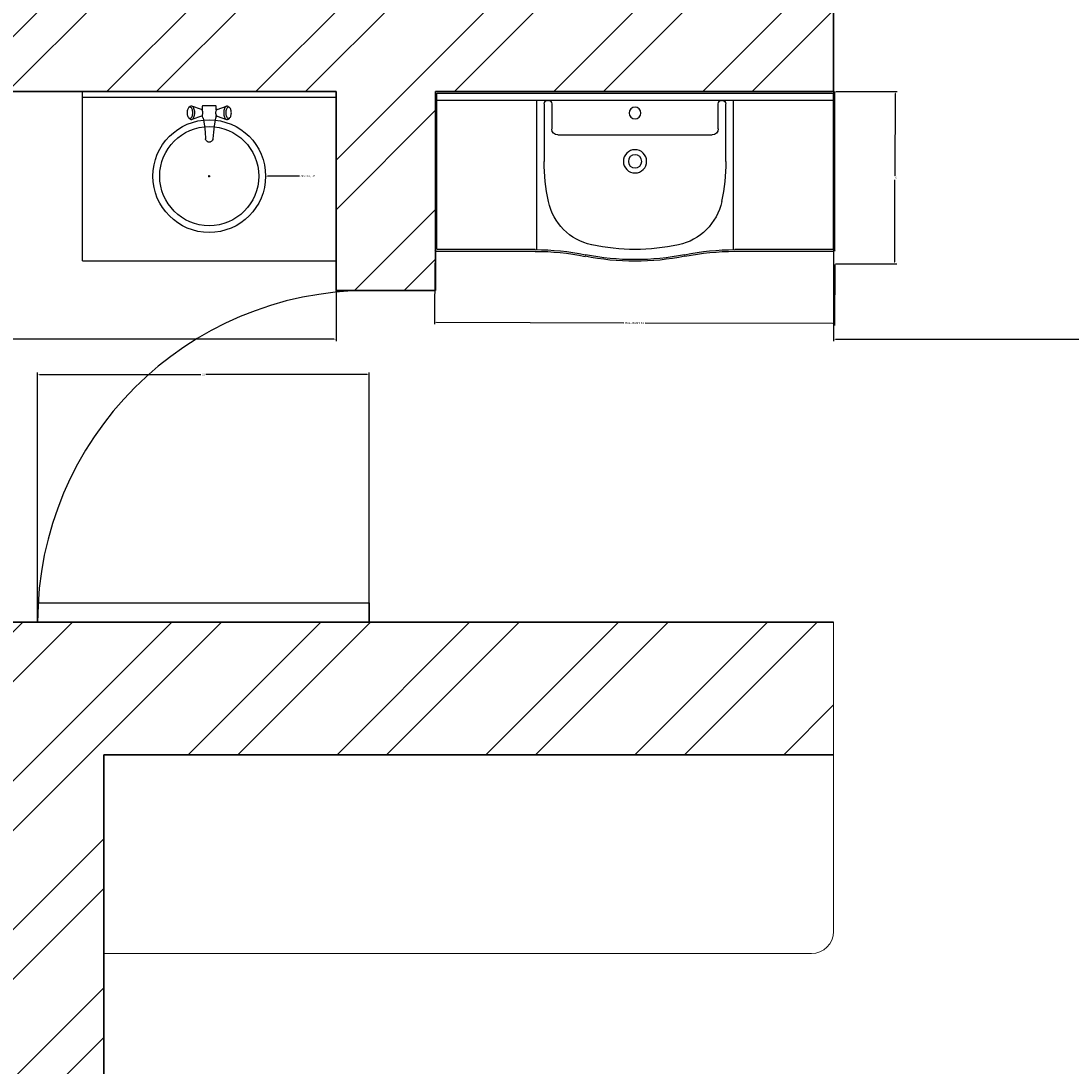
# Model space of a CAD drawing. Units: inches. Extents: x 3449 to 3843, y 1566 to 2054.
# Tile 3 of 8: x 3543 to 3638, y 1751 to 1846. Entities that reach past the tile are written whole.
import ezdxf

# ---------------------------------------------------------------- set-up
doc = ezdxf.new("R2010")
doc.units = ezdxf.units.IN
for name, color, linetype, lineweight in [('A-ANNO-DIMS', 2, 'Continuous', 18), ('A-DOOR', 4, 'Continuous', 25), ('A-FLOR-CASE', 7, 'Continuous', 20), ('A-WALL', 7, 'Continuous', 35), ('A-WALL-PATT', 251, 'Continuous', 13), ('Сантехника', 7, 'Continuous', 18)]:
    doc.layers.add(name, color=color, linetype=linetype, lineweight=lineweight)
doc.layers.add('SANTEH', color=7, linetype='Continuous')
doc.styles.get("Standard").update_dxf_attribs({"font": 'arial.ttf'})
doc.dimstyles.get("Standard").update_dxf_attribs({"dimtxt": 0.18, "dimasz": 0.18, "dimexe": 0.18, "dimexo": 0.0625, "dimgap": 0.09, "dimtad": 0, "dimtih": 1, "dimtoh": 1, "dimdec": 4, "dimzin": 0, "dimdsep": 46, "dimtxsty": 'Standard', "dimcen": 0.09, "dimadec": 0, "dimazin": 0, "dimtfac": 1, "dimtdec": 4, "dimtofl": 0, "dimtmove": 0, "dimatfit": 3, "dimfxl": 1, "dimtolj": 1, "dimtzin": 0, "dimarcsym": 0})

# ---------------------------------------------------------------- blocks, each defined once
blk = doc.blocks.new('*U6')
for p, q in [((0, 0), (0, -6)), ((30, 0), (30, -6))]:
    blk.add_line(p, q)
blk.add_lwpolyline([(0, 0), (0, 30), (1.75, 30), (1.75, 0)], close=True)
blk.add_arc((0, 0), 30, 0, 90)
blk = doc.blocks.new('Basin Built-In Circle_74')
at = {"layer": 'SANTEH'}
for p, q in [((0, 600), (900, 600)), ((0, 0), (0, 600)), ((900, 0), (900, 600)), ((0, 580), (900, 580)), ((371.7, 528.5), (371.5, 525)), ((371.7, 528.5), (371.5, 525)), ((371.5, 525), (371.7, 521.5)), ((371.5, 525), (371.7, 521.5)), ((372.1, 531.8), (371.7, 528.5)), ((372.1, 531.8), (371.7, 528.5)), ((372.8, 535), (372.1, 531.8)), ((372.8, 535), (372.1, 531.8)), ((373.8, 537.9), (372.8, 535)), ((373.8, 537.9), (372.8, 535)), ((375.1, 540.3), (373.8, 537.9)), ((375.1, 540.3), (373.8, 537.9)), ((376.5, 542.3), (375.1, 540.3)), ((376.5, 542.3), (375.1, 540.3)), ((378.1, 543.8), (376.5, 542.3)), ((378.1, 543.8), (376.5, 542.3)), ((382.6, 547.6), (378.1, 543.8)), ((382.6, 547.6), (378.1, 543.8)), ((379.8, 544.7), (378.1, 543.8)), ((379.8, 544.7), (378.1, 543.8)), ((381.5, 545), (379.8, 544.7)), ((381.5, 545), (379.8, 544.7)), ((383.2, 544.7), (381.5, 545)), ((383.2, 544.7), (381.5, 545)), ((384.6, 548.6), (382.6, 547.6)), ((384.6, 548.6), (382.6, 547.6)), ((384.9, 543.8), (383.2, 544.7)), ((384.9, 543.8), (383.2, 544.7)), ((386.7, 549), (384.6, 548.6)), ((386.7, 549), (384.6, 548.6)), ((386.5, 542.3), (384.9, 543.8)), ((386.5, 542.3), (384.9, 543.8)), ((387.9, 540.3), (386.5, 542.3)), ((387.9, 540.3), (386.5, 542.3)), ((388.8, 548.6), (386.7, 549)), ((388.8, 548.6), (386.7, 549)), ((389.2, 537.9), (387.9, 540.3)), ((389.2, 537.9), (387.9, 540.3)), ((390.8, 547.6), (388.8, 548.6)), ((422.4, 536.8), (388.8, 548.6)), ((390.8, 547.6), (388.8, 548.6)), ((422.4, 536.8), (388.8, 548.6)), ((390.2, 535), (389.2, 537.9)), ((390.2, 535), (389.2, 537.9)), ((390.9, 531.8), (390.2, 535)), ((390.9, 531.8), (390.2, 535)), ((392.7, 545.8), (390.8, 547.6)), ((392.7, 545.8), (390.8, 547.6)), ((391.4, 528.5), (390.9, 531.8)), ((391.4, 528.5), (390.9, 531.8)), ((391.5, 525), (391.4, 528.5)), ((391.5, 525), (391.4, 528.5)), ((391.4, 521.5), (391.5, 525)), ((391.4, 521.5), (391.5, 525)), ((394.4, 543.4), (392.7, 545.8)), ((394.4, 543.4), (392.7, 545.8)), ((395.9, 540.4), (394.4, 543.4)), ((395.9, 540.4), (394.4, 543.4)), ((397.1, 537), (395.9, 540.4)), ((397.1, 537), (395.9, 540.4)), ((398, 533.2), (397.1, 537)), ((398, 533.2), (397.1, 537)), ((398.5, 529.2), (398, 533.2)), ((398.5, 529.2), (398, 533.2)), ((398.7, 525), (398.5, 529.2)), ((398.7, 525), (398.5, 529.2)), ((398.5, 520.8), (398.7, 525)), ((398.5, 520.8), (398.7, 525)), ((423.4, 536.3), (422.4, 536.8)), ((423.4, 536.3), (422.4, 536.8)), ((424.3, 535.4), (423.4, 536.3)), ((424.3, 535.4), (423.4, 536.3)), ((425.2, 534.2), (424.3, 535.4)), ((425.2, 534.2), (424.3, 535.4)), ((426.7, 535), (424.6, 535)), ((426.7, 535), (424.6, 535)), ((425.2, 548), (425, 547.5)), ((425.2, 548), (425, 547.5)), ((425, 547.5), (425, 547)), ((425, 547.5), (425, 547)), ((425, 547), (425, 535)), ((425, 547), (425, 535)), ((425.4, 548.5), (425.2, 548)), ((425.4, 548.5), (425.2, 548)), ((425.9, 532.7), (425.2, 534.2)), ((425.9, 532.7), (425.2, 534.2)), ((425.7, 548.9), (425.4, 548.5)), ((425.7, 548.9), (425.4, 548.5)), ((426.1, 549.3), (425.7, 548.9)), ((426.1, 549.3), (425.7, 548.9)), ((426.5, 531), (425.9, 532.7)), ((426.5, 531), (425.9, 532.7)), ((426.5, 549.6), (426.1, 549.3)), ((426.5, 549.6), (426.1, 549.3)), ((427, 549.8), (426.5, 549.6)), ((427, 549.8), (426.5, 549.6)), ((427, 529.1), (426.5, 531)), ((427, 529.1), (426.5, 531)), ((427.5, 550), (427, 549.8)), ((427.5, 550), (427, 549.8)), ((427.2, 527.1), (427, 529.1)), ((427.2, 527.1), (427, 529.1)), ((427, 520.9), (427.2, 522.9)), ((427, 520.9), (427.2, 522.9)), ((427.3, 525), (427.2, 527.1)), ((427.3, 525), (427.2, 527.1)), ((427.2, 522.9), (427.3, 525)), ((427.2, 522.9), (427.3, 525)), ((428, 550), (427.5, 550)), ((428, 550), (427.5, 550)), ((472, 550), (428, 550)), ((472, 550), (428, 550)), ((472.5, 550), (472, 550)), ((472.5, 550), (472, 550)), ((473, 549.8), (472.5, 550)), ((473, 549.8), (472.5, 550)), ((472.8, 527.1), (472.7, 525)), ((472.8, 527.1), (472.7, 525)), ((472.7, 525), (472.8, 522.9)), ((472.7, 525), (472.8, 522.9)), ((473, 529.1), (472.8, 527.1)), ((473, 529.1), (472.8, 527.1)), ((472.8, 522.9), (473, 520.9)), ((472.8, 522.9), (473, 520.9)), ((473.5, 549.6), (473, 549.8)), ((473.5, 549.6), (473, 549.8)), ((473.5, 531), (473, 529.1)), ((473.5, 531), (473, 529.1)), ((473.9, 549.3), (473.5, 549.6)), ((473.9, 549.3), (473.5, 549.6)), ((475.4, 535), (473.5, 535)), ((475.4, 535), (473.5, 535)), ((474.1, 532.7), (473.5, 531)), ((474.1, 532.7), (473.5, 531)), ((474.3, 548.9), (473.9, 549.3)), ((474.3, 548.9), (473.9, 549.3)), ((474.8, 534.2), (474.1, 532.7)), ((474.8, 534.2), (474.1, 532.7)), ((474.6, 548.5), (474.3, 548.9)), ((474.6, 548.5), (474.3, 548.9)), ((474.8, 548), (474.6, 548.5)), ((474.8, 548), (474.6, 548.5)), ((475, 547.5), (474.8, 548)), ((475, 547.5), (474.8, 548)), ((475.7, 535.4), (474.8, 534.2)), ((475.7, 535.4), (474.8, 534.2)), ((475, 547), (475, 547.5)), ((475, 547), (475, 547.5)), ((475, 535), (475, 547)), ((475, 535), (475, 547)), ((476.6, 536.3), (475.7, 535.4)), ((476.6, 536.3), (475.7, 535.4)), ((477.6, 536.8), (476.6, 536.3)), ((477.6, 536.8), (476.6, 536.3)), ((477.6, 536.8), (511.2, 548.6)), ((477.6, 536.8), (511.2, 548.6)), ((501.5, 529.2), (501.3, 525)), ((501.5, 529.2), (501.3, 525)), ((501.3, 525), (501.5, 520.8)), ((501.3, 525), (501.5, 520.8)), ((502, 533.2), (501.5, 529.2)), ((502, 533.2), (501.5, 529.2)), ((502.9, 537), (502, 533.2)), ((502.9, 537), (502, 533.2)), ((504.1, 540.4), (502.9, 537)), ((504.1, 540.4), (502.9, 537)), ((505.6, 543.4), (504.1, 540.4)), ((505.6, 543.4), (504.1, 540.4)), ((507.3, 545.8), (505.6, 543.4)), ((507.3, 545.8), (505.6, 543.4)), ((509.2, 547.6), (507.3, 545.8)), ((509.2, 547.6), (507.3, 545.8)), ((508.6, 528.5), (508.5, 525)), ((508.6, 528.5), (508.5, 525)), ((508.5, 525), (508.6, 521.5)), ((508.5, 525), (508.6, 521.5)), ((509.1, 531.8), (508.6, 528.5)), ((509.1, 531.8), (508.6, 528.5)), ((509.8, 535), (509.1, 531.8)), ((509.8, 535), (509.1, 531.8)), ((511.2, 548.6), (509.2, 547.6)), ((511.2, 548.6), (509.2, 547.6)), ((510.8, 537.9), (509.8, 535)), ((510.8, 537.9), (509.8, 535)), ((512.1, 540.3), (510.8, 537.9)), ((512.1, 540.3), (510.8, 537.9)), ((513.3, 549), (511.2, 548.6)), ((513.3, 549), (511.2, 548.6)), ((513.5, 542.3), (512.1, 540.3)), ((513.5, 542.3), (512.1, 540.3)), ((515.4, 548.6), (513.3, 549)), ((515.4, 548.6), (513.3, 549)), ((515.1, 543.8), (513.5, 542.3)), ((515.1, 543.8), (513.5, 542.3)), ((516.8, 544.7), (515.1, 543.8)), ((516.8, 544.7), (515.1, 543.8)), ((517.4, 547.6), (515.4, 548.6)), ((517.4, 547.6), (515.4, 548.6)), ((518.5, 545), (516.8, 544.7)), ((518.5, 545), (516.8, 544.7)), ((517.4, 547.6), (521.9, 543.8)), ((517.4, 547.6), (521.9, 543.8)), ((520.2, 544.7), (518.5, 545)), ((520.2, 544.7), (518.5, 545)), ((521.9, 543.8), (520.2, 544.7)), ((521.9, 543.8), (520.2, 544.7)), ((523.5, 542.3), (521.9, 543.8)), ((523.5, 542.3), (521.9, 543.8)), ((524.9, 540.3), (523.5, 542.3)), ((524.9, 540.3), (523.5, 542.3)), ((526.2, 537.9), (524.9, 540.3)), ((526.2, 537.9), (524.9, 540.3)), ((527.2, 535), (526.2, 537.9)), ((527.2, 535), (526.2, 537.9)), ((527.9, 531.8), (527.2, 535)), ((527.9, 531.8), (527.2, 535)), ((528.3, 528.5), (527.9, 531.8)), ((528.3, 528.5), (527.9, 531.8)), ((528.5, 525), (528.3, 528.5)), ((528.5, 525), (528.3, 528.5)), ((528.3, 521.5), (528.5, 525)), ((528.3, 521.5), (528.5, 525)), ((371.7, 521.5), (372.1, 518.2)), ((371.7, 521.5), (372.1, 518.2)), ((372.1, 518.2), (372.8, 515)), ((372.1, 518.2), (372.8, 515)), ((372.8, 515), (373.8, 512.1)), ((372.8, 515), (373.8, 512.1)), ((373.8, 512.1), (375.1, 509.7)), ((373.8, 512.1), (375.1, 509.7)), ((375.1, 509.7), (376.5, 507.7)), ((375.1, 509.7), (376.5, 507.7)), ((376.5, 507.7), (378.1, 506.2)), ((376.5, 507.7), (378.1, 506.2)), ((378.1, 506.2), (379.8, 505.3)), ((382.6, 502.4), (378.1, 506.2)), ((378.1, 506.2), (379.8, 505.3)), ((382.6, 502.4), (378.1, 506.2)), ((379.8, 505.3), (381.5, 505)), ((379.8, 505.3), (381.5, 505)), ((381.5, 505), (383.2, 505.3)), ((381.5, 505), (383.2, 505.3)), ((382.6, 502.4), (384.6, 501.4)), ((382.6, 502.4), (384.6, 501.4)), ((383.2, 505.3), (384.9, 506.2)), ((383.2, 505.3), (384.9, 506.2)), ((384.6, 501.4), (386.7, 501)), ((384.6, 501.4), (386.7, 501)), ((384.9, 506.2), (386.5, 507.7)), ((384.9, 506.2), (386.5, 507.7)), ((386.5, 507.7), (387.9, 509.7)), ((386.5, 507.7), (387.9, 509.7)), ((386.7, 501), (388.8, 501.4)), ((386.7, 501), (388.8, 501.4)), ((387.9, 509.7), (389.2, 512.1)), ((387.9, 509.7), (389.2, 512.1)), ((422.4, 513.2), (388.8, 501.4)), ((422.4, 513.2), (388.8, 501.4)), ((388.8, 501.4), (390.8, 502.4)), ((388.8, 501.4), (390.8, 502.4)), ((389.2, 512.1), (390.2, 515)), ((389.2, 512.1), (390.2, 515)), ((390.2, 515), (390.9, 518.2)), ((390.2, 515), (390.9, 518.2)), ((390.8, 502.4), (392.7, 504.2)), ((390.8, 502.4), (392.7, 504.2)), ((390.9, 518.2), (391.4, 521.5)), ((390.9, 518.2), (391.4, 521.5)), ((392.7, 504.2), (394.4, 506.6)), ((392.7, 504.2), (394.4, 506.6)), ((394.4, 506.6), (395.9, 509.6)), ((394.4, 506.6), (395.9, 509.6)), ((395.9, 509.6), (397.1, 513)), ((395.9, 509.6), (397.1, 513)), ((397.1, 513), (398, 516.8)), ((397.1, 513), (398, 516.8)), ((398, 516.8), (398.5, 520.8)), ((398, 516.8), (398.5, 520.8)), ((422.4, 513.2), (423.4, 513.7)), ((422.4, 513.2), (423.4, 513.7)), ((423.4, 513.7), (424.3, 514.6)), ((423.4, 513.7), (424.3, 514.6)), ((424.3, 514.6), (425.2, 515.8)), ((424.3, 514.6), (425.2, 515.8)), ((427.1, 515), (424.6, 515)), ((427.1, 515), (424.6, 515)), ((425, 515), (425, 513)), ((425, 515), (425, 513)), ((425, 513), (425, 512.5)), ((425, 513), (425, 512.5)), ((425, 512.5), (425.2, 512)), ((425, 512.5), (425.2, 512)), ((425.2, 515.8), (425.9, 517.3)), ((425.2, 515.8), (425.9, 517.3)), ((425.2, 512), (428.1, 505.1)), ((425.2, 512), (428.1, 505.1)), ((425.9, 517.3), (426.5, 519)), ((425.9, 517.3), (426.5, 519)), ((426.5, 519), (427, 520.9)), ((426.5, 519), (427, 520.9)), ((428, 505.4), (430.7, 493.4)), ((428, 505.4), (430.7, 493.4)), ((430.7, 493.4), (433, 477.1)), ((430.7, 493.4), (433, 477.1)), ((469.3, 493.4), (467, 477.1)), ((469.3, 493.4), (467, 477.1)), ((472, 505.4), (469.3, 493.4)), ((472, 505.4), (469.3, 493.4)), ((474.8, 512), (471.9, 505.1)), ((474.8, 512), (471.9, 505.1)), ((473, 520.9), (473.5, 519)), ((473, 520.9), (473.5, 519)), ((475.4, 515), (473.2, 515)), ((475.4, 515), (473.2, 515)), ((473.5, 519), (474.1, 517.3)), ((473.5, 519), (474.1, 517.3)), ((474.1, 517.3), (474.8, 515.8)), ((474.1, 517.3), (474.8, 515.8)), ((474.8, 515.8), (475.7, 514.6)), ((474.8, 515.8), (475.7, 514.6)), ((474.8, 512), (475, 512.5)), ((474.8, 512), (475, 512.5)), ((475, 513), (475, 515)), ((475, 513), (475, 515)), ((475, 512.5), (475, 513)), ((475, 512.5), (475, 513)), ((475.7, 514.6), (476.6, 513.7)), ((475.7, 514.6), (476.6, 513.7)), ((476.6, 513.7), (477.6, 513.2)), ((476.6, 513.7), (477.6, 513.2)), ((477.6, 513.2), (511.2, 501.4)), ((477.6, 513.2), (511.2, 501.4)), ((501.5, 520.8), (502, 516.8)), ((501.5, 520.8), (502, 516.8)), ((502, 516.8), (502.9, 513)), ((502, 516.8), (502.9, 513)), ((502.9, 513), (504.1, 509.6)), ((502.9, 513), (504.1, 509.6)), ((504.1, 509.6), (505.6, 506.6)), ((504.1, 509.6), (505.6, 506.6)), ((505.6, 506.6), (507.3, 504.2)), ((505.6, 506.6), (507.3, 504.2)), ((507.3, 504.2), (509.2, 502.4)), ((507.3, 504.2), (509.2, 502.4)), ((508.6, 521.5), (509.1, 518.2)), ((508.6, 521.5), (509.1, 518.2)), ((509.1, 518.2), (509.8, 515)), ((509.1, 518.2), (509.8, 515)), ((509.2, 502.4), (511.2, 501.4)), ((509.2, 502.4), (511.2, 501.4)), ((509.8, 515), (510.8, 512.1)), ((509.8, 515), (510.8, 512.1)), ((510.8, 512.1), (512.1, 509.7)), ((510.8, 512.1), (512.1, 509.7)), ((511.2, 501.4), (513.3, 501)), ((511.2, 501.4), (513.3, 501)), ((512.1, 509.7), (513.5, 507.7)), ((512.1, 509.7), (513.5, 507.7)), ((513.3, 501), (515.4, 501.4)), ((513.3, 501), (515.4, 501.4)), ((513.5, 507.7), (515.1, 506.2)), ((513.5, 507.7), (515.1, 506.2)), ((515.1, 506.2), (516.8, 505.3)), ((515.1, 506.2), (516.8, 505.3)), ((515.4, 501.4), (517.4, 502.4)), ((515.4, 501.4), (517.4, 502.4)), ((516.8, 505.3), (518.5, 505)), ((516.8, 505.3), (518.5, 505)), ((517.4, 502.4), (521.9, 506.2)), ((517.4, 502.4), (521.9, 506.2)), ((518.5, 505), (520.2, 505.3)), ((518.5, 505), (520.2, 505.3)), ((520.2, 505.3), (521.9, 506.2)), ((520.2, 505.3), (521.9, 506.2)), ((521.9, 506.2), (523.5, 507.7)), ((521.9, 506.2), (523.5, 507.7)), ((523.5, 507.7), (524.9, 509.7)), ((523.5, 507.7), (524.9, 509.7)), ((524.9, 509.7), (526.2, 512.1)), ((524.9, 509.7), (526.2, 512.1)), ((526.2, 512.1), (527.2, 515)), ((526.2, 512.1), (527.2, 515)), ((527.2, 515), (527.9, 518.2)), ((527.2, 515), (527.9, 518.2)), ((527.9, 518.2), (528.3, 521.5)), ((527.9, 518.2), (528.3, 521.5)), ((433, 477.2), (435, 456.1)), ((433, 477.2), (435, 456.1)), ((435, 456.1), (436.8, 432.9)), ((435, 456.1), (436.8, 432.9)), ((465, 456.1), (463.2, 432.9)), ((465, 456.1), (463.2, 432.9)), ((467, 477.2), (465, 456.1)), ((467, 477.2), (465, 456.1)), ((437, 430.8), (436.8, 432.9)), ((437, 430.8), (436.8, 432.9)), ((437, 430.7), (437, 430.8)), ((437, 430.7), (437, 430.8)), ((437.6, 428.7), (437, 430.7)), ((437.6, 428.7), (437, 430.7)), ((438.6, 426.9), (437.6, 428.7)), ((438.6, 426.9), (437.6, 428.7)), ((440, 425.1), (438.6, 426.9)), ((440, 425.1), (438.6, 426.9)), ((441.6, 423.7), (440, 425.1)), ((441.6, 423.7), (440, 425.1)), ((443.5, 422.5), (441.6, 423.7)), ((443.5, 422.5), (441.6, 423.7)), ((445.6, 421.7), (443.5, 422.5)), ((445.6, 421.7), (443.5, 422.5)), ((445, 421.7), (443.9, 422.4)), ((446.6, 421), (445, 421.7)), ((447.7, 421.2), (445.6, 421.7)), ((447.7, 421.2), (445.6, 421.7)), ((448.3, 420.6), (446.6, 421)), ((450, 421), (447.7, 421.2)), ((450, 421), (447.7, 421.2)), ((450, 420.5), (448.3, 420.6)), ((452.3, 421.2), (450, 421)), ((452.3, 421.2), (450, 421)), ((451.7, 420.6), (450, 420.5)), ((453.4, 421), (451.7, 420.6)), ((454.4, 421.7), (452.3, 421.2)), ((454.4, 421.7), (452.3, 421.2)), ((455, 421.7), (453.4, 421)), ((456.5, 422.5), (454.4, 421.7)), ((456.5, 422.5), (454.4, 421.7)), ((456.1, 422.4), (455, 421.7)), ((458.4, 423.7), (456.5, 422.5)), ((458.4, 423.7), (456.5, 422.5)), ((460, 425.1), (458.4, 423.7)), ((460, 425.1), (458.4, 423.7)), ((461.4, 426.9), (460, 425.1)), ((461.4, 426.9), (460, 425.1)), ((462.4, 428.7), (461.4, 426.9)), ((462.4, 428.7), (461.4, 426.9)), ((463, 430.7), (462.4, 428.7)), ((463, 430.7), (462.4, 428.7)), ((463.2, 432.9), (463, 430.8)), ((463.2, 432.9), (463, 430.8)), ((463, 430.7), (463, 430.8)), ((463, 430.7), (463, 430.8)), ((0, 0), (900, 0))]:
    blk.add_line(p, q, dxfattribs=at)
for radius in [200, 175.8]:
    blk.add_circle((450, 300), radius, dxfattribs=at)
blk = doc.blocks.new('s_02')
at = {"layer": 'SANTEH'}
for p, q in [((0, 0), (-519.4, -1.7)), ((0, 0), (-519.4, -1.7)), ((-520.5, -2.8), (-519.8, -209.5)), ((-520.5, -2.8), (-519.8, -209.5)), ((-517.6, -207.3), (-518.3, -5)), ((-1, -11.7), (-518.3, -13.5)), ((-517.2, -3.9), (-2.2, -2.2)), ((-387.2, -207.9), (-387.9, -13)), ((-131.4, -12.2), (-130.8, -207.1)), ((-1.1, -3.3), (-0.4, -205.6)), ((1.8, -207.7), (1.1, -1.1)), ((1.8, -207.7), (1.1, -1.1)), ((-378.3, -17.4), (-378.1, -92.6)), ((-368.3, -17.3), (-368.2, -50.3)), ((-150.9, -49.6), (-151, -16.6)), ((-140.7, -91.8), (-141, -16.6)), ((-360.4, -58.1), (-158.7, -57.4)), ((-518.7, -210.5), (-389.4, -210.1)), ((-518.7, -210.5), (-389.4, -210.1)), ((-389.4, -207.9), (-516.6, -208.4)), ((-1.5, -206.6), (-128.6, -207.1)), ((-128.6, -209.2), (0.7, -208.8)), ((-128.6, -209.2), (0.7, -208.8))]:
    blk.add_line(p, q, dxfattribs=at)
at = {"layer": 'SANTEH', "extrusion": (0, 0, -1)}
for centre, major_axis, ratio, start_param, end_param in [((0, -1.1), (-0.38, 1.02), 0.991976, 0.357514, 1.923061), ((0, -1.1), (-0.38, 1.02), 0.991976, 0.357514, 1.923061), ((-519.4, -2.8), (0, -1.09), 0.99914, 1.570796, 3.141593), ((-519.4, -2.8), (0, -1.09), 0.99914, 1.570796, 3.141593), ((-517.2, -5), (0, -1.09), 0.99914, 1.570796, 3.141593), ((-374, -17.3), (0.01, -4.35), 0.99914, 1.570796, 3.141593), ((-372.7, -17.3), (0.01, -4.35), 0.99914, 3.141593, 4.712389), ((-146.6, -16.6), (0.01, -4.35), 0.99914, 1.570796, 3.141593), ((-145.3, -16.6), (0.01, -4.35), 0.99914, 3.141593, 4.712389), ((-2.2, -3.3), (0, -1.09), 0.99914, 3.141593, 4.712389), ((-259.6, -29.1), (0.03, -7.61), 0.99914, 1.570796326742688, 7.853981633922275), ((-360.4, -50.3), (0.03, -7.83), 0.99914, 0, 1.570796), ((-158.7, -49.6), (0.03, -7.83), 0.99914, -1.570796, 0), ((-259.4, -92.2), (0.1, -15.2), 0.99914, 1.570796326791235, 7.853981633970821), ((-128, -91.8), (0.8, -250.2), 0.99914, 1.359365, 1.570796), ((-259.4, -92.2), (0.03, -8.7), 0.99914, 1.570796326873691, 7.853981634053277), ((-390.8, -92.7), (0.8, -250.2), 0.99914, -1.570796, -1.359365), ((-300.4, -129.4), (0.2, -73.7), 0.99914, 0.211723, 1.359365), ((-218.1, -129.1), (0.2, -73.7), 0.99914, -1.359365, -0.211723), ((-259.9, 62.3), (0.9, -269.6), 0.99914, -0.211723, 0.211723), ((-1.5, -205.6), (0, -1.09), 0.99914, 4.712389, 6.283185), ((-518.7, -209.5), (0, -1.09), 0.99914, 0, 1.570796), ((-518.7, -209.5), (0, -1.09), 0.99914, 0, 1.570796), ((-516.6, -207.3), (0, -1.09), 0.99914, 0, 1.570796), ((-388.3, -539.7), (1.1, -331.7), 0.99914, 3.141593, 3.34093), ((-388.3, -539.7), (1.1, -329.5), 0.99914, 3.141593, 3.34093), ((-388.3, -539.7), (1.1, -329.5), 0.99914, 3.141593, 3.34093), ((-260.1, 106.8), (1.1, -329.5), 0.99914, -0.199337, 0.199337), ((-260.1, 106.8), (1.1, -329.5), 0.99914, -0.199337, 0.199337), ((-260.1, 106.8), (1.1, -327.4), 0.99914, -0.199337, 0.199337), ((-127.5, -538.8), (1.1, -331.7), 0.99914, 2.942255, 3.141593), ((-127.5, -538.8), (1.1, -329.5), 0.99914, 2.942255, 3.141593), ((-127.5, -538.8), (1.1, -329.5), 0.99914, 2.942255, 3.141593), ((0.7, -207.7), (0, -1.09), 0.99914, 4.712389, 6.283185), ((0.7, -207.7), (0, -1.09), 0.99914, 4.712389, 6.283185)]:
    blk.add_ellipse(centre, major_axis=major_axis, ratio=ratio, start_param=start_param, end_param=end_param, dxfattribs=at)
blk = doc.blocks.new('*D64')
at = {"layer": 'A-ANNO-DIMS', "color": 0, "lineweight": -2, "transparency": 16777216}
for p, q in [((3580.014, 1824.107), (3579.996, 1818.561)), ((3616.2, 1823.986), (3616.181, 1818.441)), ((3580.176, 1818.741), (3597.113, 1818.684)), ((3616.002, 1818.621), (3599.065, 1818.678))]:
    blk.add_line(p, q, dxfattribs=at)
at = {"layer": 'A-ANNO-DIMS', "color": 0, "transparency": 16777216}
for points in [[(3580.177, 1818.771), (3580.176, 1818.711), (3579.996, 1818.741)], [(3616.002, 1818.651), (3616.002, 1818.591), (3616.182, 1818.621)]]:
    blk.add_solid(points, dxfattribs=at)
at = {"layer": 'Defpoints', "color": 0, "transparency": 16777216}
for p in [(3580.015, 1824.169), (3616.2, 1824.048), (3616.182, 1818.621)]:
    blk.add_point(p, dxfattribs=at)
at = {"layer": 'A-ANNO-DIMS', "color": 0, "transparency": 16777216, "insert": (3598.089, 1818.681), "char_height": 0.18, "attachment_point": 5}
blk.add_mtext('\\A1;HALL BASIN 36', dxfattribs=at)
blk = doc.blocks.new('*D65')
at = {"layer": 'A-ANNO-DIMS', "color": 0, "lineweight": -2, "transparency": 16777216}
for p, q in [((3616.314, 1839.636), (3621.86, 1839.617)), ((3621.679, 1839.438), (3621.654, 1832.006)), ((3621.628, 1824.21), (3621.653, 1831.642)), ((3616.262, 1824.048), (3621.808, 1824.03))]:
    blk.add_line(p, q, dxfattribs=at)
at = {"layer": 'A-ANNO-DIMS', "color": 0, "transparency": 16777216}
for points in [[(3621.649, 1839.438), (3621.709, 1839.438), (3621.68, 1839.618)], [(3621.598, 1824.21), (3621.658, 1824.21), (3621.628, 1824.03)]]:
    blk.add_solid(points, dxfattribs=at)
at = {"layer": 'Defpoints', "color": 0, "transparency": 16777216}
for p in [(3616.252, 1839.636), (3621.68, 1839.618), (3616.2, 1824.048)]:
    blk.add_point(p, dxfattribs=at)
at = {"layer": 'A-ANNO-DIMS', "color": 0, "transparency": 16777216, "insert": (3621.654, 1831.824), "char_height": 0.18, "attachment_point": 5}
blk.add_mtext('\\A1;16', dxfattribs=at)
blk = doc.blocks.new('*D89')
at = {"layer": 'A-ANNO-DIMS', "color": 0, "lineweight": -2, "transparency": 16777216}
for p, q in [((3481.088, 1839.552), (3481.088, 1817.034)), ((3571.088, 1839.552), (3571.088, 1817.034)), ((3481.268, 1817.214), (3525.869, 1817.214)), ((3570.908, 1817.214), (3526.307, 1817.214))]:
    blk.add_line(p, q, dxfattribs=at)
at = {"layer": 'A-ANNO-DIMS', "color": 0, "transparency": 16777216}
for points in [[(3481.268, 1817.244), (3481.268, 1817.184), (3481.088, 1817.214)], [(3570.908, 1817.244), (3570.908, 1817.184), (3571.088, 1817.214)]]:
    blk.add_solid(points, dxfattribs=at)
at = {"layer": 'Defpoints', "color": 0, "transparency": 16777216}
for p in [(3481.088, 1839.614), (3571.088, 1839.614), (3481.088, 1817.214)]:
    blk.add_point(p, dxfattribs=at)
at = {"layer": 'A-ANNO-DIMS', "color": 0, "transparency": 16777216, "insert": (3526.088, 1817.214), "char_height": 0.18, "attachment_point": 5}
blk.add_mtext('\\A1;90', dxfattribs=at)
blk = doc.blocks.new('*D94')
at = {"layer": 'A-ANNO-DIMS', "color": 0, "lineweight": -2, "transparency": 16777216}
for p, q in [((3616.088, 1839.552), (3616.088, 1817.034)), ((3664.088, 1839.552), (3664.088, 1817.034)), ((3616.268, 1817.214), (3639.865, 1817.214)), ((3663.908, 1817.214), (3640.311, 1817.214))]:
    blk.add_line(p, q, dxfattribs=at)
at = {"layer": 'A-ANNO-DIMS', "color": 0, "transparency": 16777216}
for points in [[(3616.268, 1817.244), (3616.268, 1817.184), (3616.088, 1817.214)], [(3663.908, 1817.244), (3663.908, 1817.184), (3664.088, 1817.214)]]:
    blk.add_solid(points, dxfattribs=at)
at = {"layer": 'Defpoints', "color": 0, "transparency": 16777216}
for p in [(3616.088, 1839.614), (3664.088, 1839.614), (3616.088, 1817.214)]:
    blk.add_point(p, dxfattribs=at)
at = {"layer": 'A-ANNO-DIMS', "color": 0, "transparency": 16777216, "insert": (3640.088, 1817.214), "char_height": 0.18, "attachment_point": 5}
blk.add_mtext('\\A1;48', dxfattribs=at)
blk = doc.blocks.new('*D111')
at = {"layer": 'A-ANNO-DIMS', "color": 0, "lineweight": -2, "transparency": 16777216}
for p, q in [((3544.088, 1791.677), (3544.088, 1814.194)), ((3544.268, 1814.014), (3558.869, 1814.014)), ((3573.908, 1814.014), (3559.307, 1814.014)), ((3574.088, 1791.677), (3574.088, 1814.194))]:
    blk.add_line(p, q, dxfattribs=at)
at = {"layer": 'A-ANNO-DIMS', "color": 0, "transparency": 16777216}
for points in [[(3544.268, 1814.044), (3544.268, 1813.984), (3544.088, 1814.014)], [(3573.908, 1814.044), (3573.908, 1813.984), (3574.088, 1814.014)]]:
    blk.add_solid(points, dxfattribs=at)
at = {"layer": 'Defpoints', "color": 0, "transparency": 16777216}
for p in [(3574.088, 1814.014), (3544.088, 1791.614), (3574.088, 1791.614)]:
    blk.add_point(p, dxfattribs=at)
at = {"layer": 'A-ANNO-DIMS', "color": 0, "transparency": 16777216, "insert": (3559.088, 1814.014), "char_height": 0.18, "attachment_point": 5}
blk.add_mtext('\\A1;30', dxfattribs=at)
blk = doc.blocks.new('*D127')
at = {"layer": 'A-ANNO-DIMS', "color": 0, "lineweight": -2, "transparency": 16777216}
for p, q in [((3559.527, 1831.967), (3559.707, 1831.967)), ((3559.617, 1831.877), (3559.617, 1832.057)), ((3567.774, 1831.967), (3564.895, 1831.967))]:
    blk.add_line(p, q, dxfattribs=at)
at = {"layer": 'A-ANNO-DIMS', "color": 0, "transparency": 16777216}
blk.add_solid([(3564.895, 1831.997), (3564.895, 1831.937), (3564.715, 1831.967)], dxfattribs=at)
at = {"layer": 'Defpoints', "color": 0, "transparency": 16777216}
for p in [(3554.518, 1831.967), (3564.715, 1831.967)]:
    blk.add_point(p, dxfattribs=at)
at = {"layer": 'A-ANNO-DIMS', "color": 0, "transparency": 16777216, "insert": (3568.526, 1831.967), "char_height": 0.18, "attachment_point": 5}
blk.add_mtext('\\A1;2X ∅10.197', dxfattribs=at)

msp = doc.modelspace()

# ---------------------------------------------------------------- hatches: boundary and pattern name
at = {"layer": 'A-WALL-PATT'}
h = msp.add_hatch(dxfattribs=at)
h.set_pattern_fill('ANSI32', color=256)
edge = h.paths.add_edge_path()
edge.add_line((3481.088, 2022.6144), (3508.088, 2022.6144))
edge.add_line((3508.088, 2022.6144), (3508.088, 2031.6144))
edge.add_line((3508.088, 2031.6144), (3472.088, 2031.6144))
edge.add_line((3472.088, 2031.6144), (3472.088, 1779.6144))
edge.add_line((3472.088, 1779.6144), (3481.088, 1779.6144))
edge.add_line((3481.088, 1779.6144), (3481.088, 1839.6144))
edge.add_line((3481.088, 1839.6144), (3571.088, 1839.6144))
edge.add_line((3571.088, 1839.6144), (3571.088, 1824.3194))
edge.add_line((3571.088, 1824.3194), (3571.088, 1821.6144))
edge.add_line((3571.088, 1821.6144), (3580.088, 1821.6144))
edge.add_line((3580.088, 1821.6144), (3580.088, 1825.1908))
edge.add_ellipse((3580.1411, 1825.2442), major_axis=(0, 0.0754), ratio=0.9991395, start_angle=90, end_angle=135.183195, ccw=False)
edge.add_line((3580.0017, 1825.3196), (3580.0658, 1825.3196))
edge.add_line((3580.0658, 1825.3196), (3580.066, 1839.6365))
edge.add_line((3580.066, 1839.6365), (3616.088, 1839.6365))
edge.add_line((3616.088, 1839.6365), (3616.088, 1848.6144))
edge.add_line((3616.088, 1848.6144), (3610.088, 1848.6144))
edge.add_line((3610.088, 1848.6144), (3574.088, 1848.6144))
edge.add_line((3574.088, 1848.6144), (3481.088, 1848.6144))
edge.add_line((3481.088, 1848.6144), (3481.088, 1872.6144))
edge.add_line((3481.088, 1872.6144), (3481.088, 2022.6144))
h.paths.add_polyline_path([(3550.088, 1779.6144), (3616.088, 1779.6144), (3616.088, 1791.6144), (3505.088, 1791.6144), (3505.088, 1779.6144), (3541.088, 1779.6144), (3541.088, 1657.6144), (3481.088, 1657.6144), (3481.088, 1588.6144), (3496.088, 1588.6144), (3496.088, 1594.6144), (3496.088, 1597.6144), (3490.088, 1597.6144), (3490.088, 1648.6144), (3550.088, 1648.6144)])
h.paths.add_polyline_path([(3775.088, 1612.6144), (3766.088, 1612.6144), (3766.088, 1597.6144), (3536.088, 1597.6144), (3536.088, 1588.6144), (3775.088, 1588.6144)])
h.paths.add_polyline_path([(3820.088, 1756.6144), (3811.088, 1756.6144), (3811.088, 1732.6144), (3664.088, 1732.6144), (3664.088, 1723.6144), (3766.088, 1723.6144), (3766.088, 1708.6144), (3775.088, 1708.6144), (3775.088, 1723.6144), (3820.088, 1723.6144)])
h.paths.add_polyline_path([(3820.088, 1986.6144), (3745.088, 1986.6144), (3745.088, 2010.6144), (3664.088, 2010.6144), (3664.088, 1992.6144), (3652.088, 1992.6144), (3652.088, 1983.6144), (3664.088, 1983.6144), (3664.088, 1893.6144), (3648.793, 1893.6144), (3607.088, 1893.6144), (3607.088, 1884.6144), (3673.088, 1884.6144), (3673.088, 2001.6144), (3736.088, 2001.6144), (3736.088, 1977.6144), (3811.088, 1977.6144), (3811.088, 1949.1144), (3820.088, 1949.1144)])
h.paths.add_polyline_path([(3628.088, 1992.6144), (3616.088, 1992.6144), (3616.088, 2031.6144), (3580.088, 2031.6144), (3580.088, 2022.6144), (3607.088, 2022.6144), (3607.088, 1921.6144), (3613.088, 1921.6144), (3616.088, 1921.6144), (3616.088, 1983.6144), (3628.088, 1983.6144)])
h.paths.add_polyline_path([(3820.088, 1877.1144), (3811.088, 1877.1144), (3811.088, 1848.6144), (3664.088, 1848.6144), (3664.088, 1839.6144), (3700.088, 1839.6144), (3811.088, 1839.6144), (3811.088, 1815.6144), (3820.088, 1815.6144)])

# ---------------------------------------------------------------- linework, layer by layer
at = {"layer": 'A-FLOR-CASE'}
for p, q in [((3616.088, 1791.6144), (3616.088, 1763.6144)), ((3550.088, 1761.6144), (3614.088, 1761.6144))]:
    msp.add_line(p, q, dxfattribs=at)
msp.add_arc((3614.088, 1763.6144), 2, 270, 0, dxfattribs=at)
at = {"layer": 'A-WALL'}
for p, q in [((3616.088, 1848.6144), (3616.088, 1839.6144)), ((3481.088, 1839.6144), (3571.088, 1839.6144)), ((3571.088, 1839.6144), (3571.088, 1821.6144)), ((3580.088, 1839.6144), (3580.088, 1821.6144)), ((3580.088, 1839.6144), (3616.088, 1839.6144)), ((3571.088, 1821.6144), (3580.088, 1821.6144)), ((3481.088, 1791.6144), (3616.088, 1791.6144)), ((3550.088, 1779.6144), (3550.088, 1648.6144)), ((3550.088, 1779.6144), (3616.088, 1779.6144))]:
    msp.add_line(p, q, dxfattribs=at)

# ---------------------------------------------------------------- block references
at = {"layer": 'A-DOOR', "rotation": 90}
msp.add_blockref('*U6', (3574.088, 1791.6144), dxfattribs=at)
at = {"layer": 'Сантехника', "ltscale": 5, "xscale": 0.0254916274909978, "yscale": 0.0254916274909978, "zscale": 0.0254916274909978}
msp.add_blockref('Basin Built-In Circle_74', (3548.1456, 1824.3194), dxfattribs=at)
at = {"layer": 'Сантехника', "xscale": 0.0692834024604046, "yscale": 0.0692834024604046, "zscale": 0.0692834024604046, "rotation": 359.8089999999223}
msp.add_blockref('s_02', (3616.1286, 1839.6361), dxfattribs=at)

# ---------------------------------------------------------------- dimensions: what is measured, and where the dimension line sits
at = {"layer": 'A-ANNO-DIMS'}
for base, p1, p2, angle, picture, middle in [((3481.088, 1817.2144), (3571.088, 1839.6144), (3481.088, 1839.6144), 180, '*D89', (3526.088, 1817.2144)), ((3616.088, 1817.2144), (3664.088, 1839.6144), (3616.088, 1839.6144), 180, '*D94', (3640.088, 1817.2144)), ((3621.6797, 1839.618), (3616.1999, 1824.0484), (3616.2519, 1839.6361), 89.809, '*D65', (3621.6537, 1831.8241))]:
    dim = msp.add_linear_dim(base=base, p1=p1, p2=p2, angle=angle, dimstyle='Standard', override={"dimdec": 0, "dimlfac": 1, "dimrnd": 0, "dimzin": 0, "dimdsep": 46, "dimlunit": 2}, dxfattribs=at)
    dim.commit()
    dim.dimension.update_dxf_attribs({"geometry": picture, "text_midpoint": middle})
dim = msp.add_diameter_dim_2p(p1=(3554.5185, 1831.9668), p2=(3564.7151, 1831.967), text='2X <>', dimstyle='Standard', override={"dimdec": 3, "dimlfac": 1, "dimrnd": 0, "dimzin": 0, "dimdsep": 46, "dimlunit": 2}, dxfattribs=at)
dim.commit()
dim.dimension.update_dxf_attribs({"geometry": '*D127', "text_midpoint": (3567.7741, 1831.9671), "dimtype": 163})
dim = msp.add_linear_dim(base=(3616.1818, 1818.6206), p1=(3580.0145, 1824.169), p2=(3616.1999, 1824.0484), angle=359.809, text='HALL BASIN <>', dimstyle='Standard', override={"dimdec": 0, "dimlfac": 1, "dimrnd": 0, "dimzin": 0, "dimdsep": 46, "dimlunit": 2}, dxfattribs=at)
dim.commit()
dim.dimension.update_dxf_attribs({"geometry": '*D64', "text_midpoint": (3598.0891, 1818.6809)})
dim = msp.add_linear_dim(base=(3574.088, 1814.0144), p1=(3544.088, 1791.6144), p2=(3574.088, 1791.6144), dimstyle='Standard', override={"dimdec": 0, "dimlfac": 1, "dimrnd": 0, "dimzin": 0, "dimdsep": 46, "dimlunit": 2}, dxfattribs=at)
dim.commit()
dim.dimension.update_dxf_attribs({"geometry": '*D111', "text_midpoint": (3559.088, 1814.0144)})

doc.saveas('drawing.dxf')
